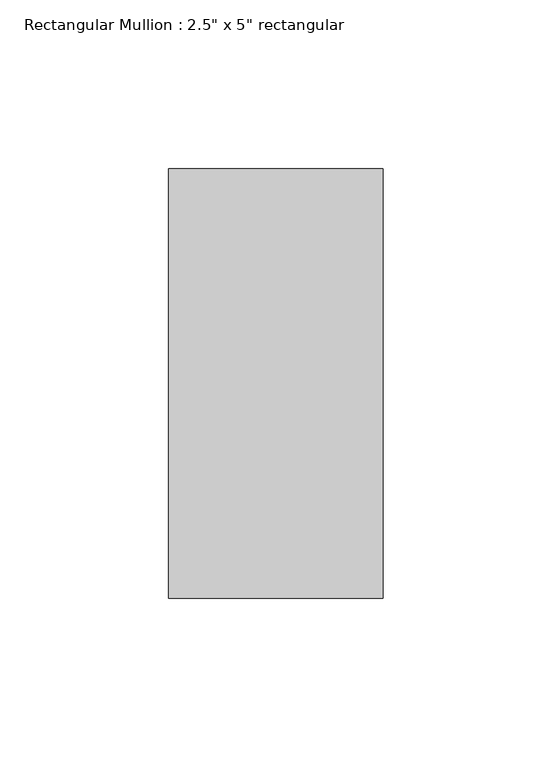
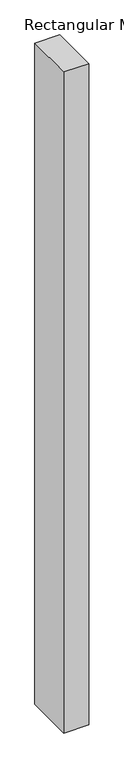
"""IFC4 building model written with IfcOpenShell, lengths in millimetres: member geometry."""

from ifc_helpers import new_model, si_unit, frame, origin, place, context, project, spatial, polyline, outline, extrude, source, transform, mapped, element, save


def member_58f5e783(model_context):
    return source(origin(), model_context, "Body", "SweptSolid", [
        extrude(outline(polyline([(31.75, 63.5), (31.75, -63.5), (-31.75, -63.5), (-31.75, 63.5), (31.75, 63.5)])), frame((0.0, 0.0, -1779.2221241), z_axis=(0.0, 0.0, 1.0), x_axis=(1.0, 0.0, 0.0)), (0.0, 0.0, 1.0), 1779.2221241),
    ])


if __name__ == "__main__":
    model = new_model("IFC4")
    model_context = context("Model", 3, world=origin())
    ifc_project = project(units=[si_unit("LENGTHUNIT", "METRE", prefix="MILLI")], contexts=[model_context])
    site = spatial("IfcSite", under=ifc_project)
    building = spatial("IfcBuilding", under=site)
    placement = place(None, origin())
    member_shape = member_58f5e783(model_context)
    element("IfcMember", 1, ObjectType="Rectangular Mullion : 2.5\" x 5\" rectangular", at=placement, inside=building, context=model_context, shape_type="MappedRepresentation", body=[
        mapped(member_shape, transform((0.0, 0.0, 0.0), x_axis=(1.0, 0.0, 0.0), y_axis=(0.0, 1.0, 0.0), z_axis=(0.0, 0.0, 1.0))),
    ])
    save(model, "model.ifc")

# Revit data of these elements
# Type "Rectangular Mullion : 2.5\" x 5\" rectangular"
#   built-in parameter 1007304 = 0.416667 (stored number, unit not read)
#   built-in parameter 1007301 = 0.104167 (stored number, unit not read)
#   built-in parameter 1007300 = 0.104167 (stored number, unit not read)
# Element 1 (IfcMember, "Rectangular Mullion : 2.5\" x 5\" rectangular")
#   Materials on its faces: "Aluminum"
# Materials
#   "Aluminum": class "Metal", colour RGB 247 247 247, transparency 0, Description = "Aluminum 6061", Cost = 0
